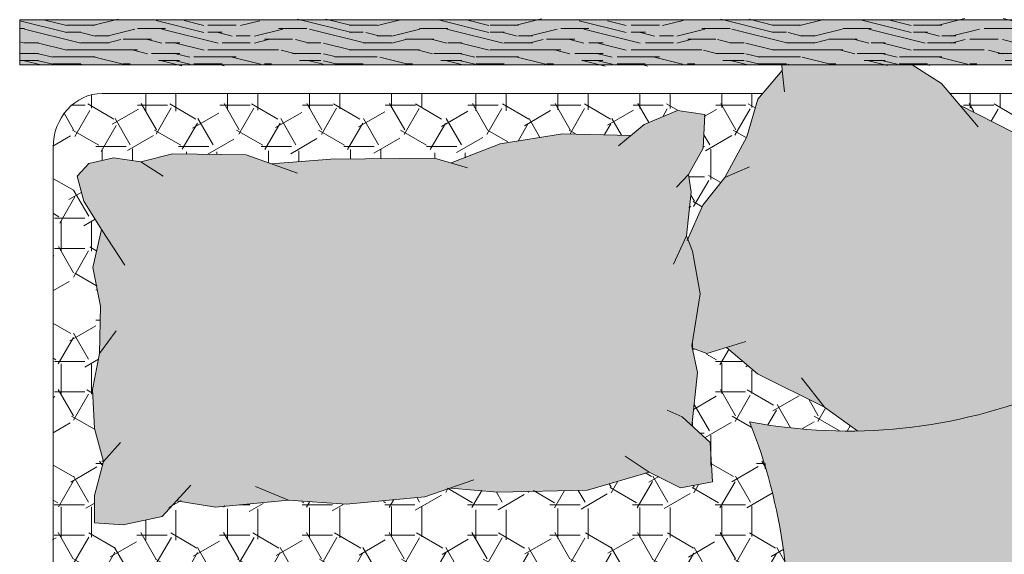
# Model space of a CAD drawing. Units: inches. Extents: x 1994 to 3075, y 3517 to 3950.
# Tile 44 of 58: x 1994.62902 to 1994.66748, y 3553.75542 to 3553.77632. Entities that reach past the tile are written whole.
import ezdxf

# ---------------------------------------------------------------- set-up
doc = ezdxf.new("R2010")
doc.units = ezdxf.units.IN
doc.layers.add('A-FURN-REFR', color=8, linetype='Continuous', lineweight=13)
doc.layers.add('A-FURN-REFR-PATT', color=8, linetype='Continuous', lineweight=13)

msp = doc.modelspace()

# ---------------------------------------------------------------- hatches: boundary and pattern name
at = {"layer": 'A-FURN-REFR-PATT'}
msp.add_hatch(color=256, dxfattribs=at).paths.add_polyline_path([(1994.683555, 3553.776316), (1994.629017, 3553.776316), (1994.629017, 3553.774549), (1994.683555, 3553.774549)])
h = msp.add_hatch(dxfattribs=at)
h.set_pattern_fill('LEGNO1', color=256, scale=0.005512, style=0, pattern_type=2)
h.set_pattern_definition([(0, (2000.7131367, 3549.9540566), (0, 0.005511811), [0.0011023622, -0.0016535433, 0.000551181, -0.0022047244]), (0, (2000.716995, 3549.9541944), (0, 0.005511811), [0.001102362, -0.004409449]), (0, (2000.716444, 3549.95447), (0, 0.005511811), [0.000551181, -0.00496063]), (0, (2000.713412, 3549.954608), (0, 0.005511811), [0.0002755906, -0.0038582677, 0.0002755906, -0.0011023622]), (0, (2000.7153414, 3549.9548834), (0, 0.005511811), [0.0011023622, -0.0016535433, 0.0002755906, -0.002480315]), (0, (2000.7139634, 3549.955021), (0, 0.005511811), [0.0008267717, -0.0046850394]), (0, (2000.7153414, 3549.955159), (0, 0.005511811), [0.0016535433, -0.0038582677]), (0, (2000.713688, 3549.955297), (0, 0.005511811), [0.001102362, -0.004409449]), (0, (2000.7158926, 3549.9554346), (0, 0.005511811), [0.0027559055, -0.0027559055]), (0, (2000.714239, 3549.95571), (0, 0.005511811), [0.000551181, -0.0016535433, 0.0011023622, -0.0022047244]), (0, (2000.7180973, 3549.955848), (0, 0.005511811), [0.001102362, -0.004409449]), (0, (2000.716995, 3549.955986), (0, 0.005511811), [0.000551181, -0.00496063]), (0, (2000.7158926, 3549.9561236), (0, 0.005511811), [0.000551181, -0.00496063]), (0, (2000.7131367, 3549.9562614), (0, 0.005511811), [0.001102362, -0.004409449]), (0, (2000.7158926, 3549.956399), (0, 0.005511811), [0.001102362, -0.004409449]), (0, (2000.7158926, 3549.956675), (0, 0.005511811), [0.0011023622, -0.0011023622, 0.0011023622, -0.0022047244]), (0, (2000.71479, 3549.9569503), (0, 0.005511811), [0.000551181, -0.0027559055, 0.0011023622, -0.0011023622]), (0, (2000.7158926, 3549.957088), (0, 0.005511811), [0.0016535433, -0.0038582677]), (0, (2000.7158926, 3549.957364), (0, 0.005511811), [0.001102362, -0.004409449]), (0, (2000.713688, 3549.9575015), (0, 0.005511811), [0.0016535433, -0.0022047244, 0.000551181, -0.0011023622]), (0, (2000.713688, 3549.957777), (0, 0.005511811), [0.0027559055, -0.0027559055]), (0, (2000.716995, 3549.957915), (0, 0.005511811), [0.000551181, -0.00496063]), (0, (2000.7153414, 3549.9580527), (0, 0.005511811), [0.001102362, -0.004409449]), (0, (2000.714239, 3549.9581905), (0, 0.005511811), [0.000551181, -0.0022047244, 0.000551181, -0.0022047244]), (0, (2000.713688, 3549.9583283), (0, 0.005511811), [0.000551181, -0.0016535433, 0.0011023622, -0.0022047244]), (0, (2000.71479, 3549.958466), (0, 0.005511811), [0.000551181, -0.0027559055, 0.000551181, -0.0016535433]), (0, (2000.7158926, 3549.958604), (0, 0.005511811), [0.0016535433, -0.0038582677]), (0, (2000.713688, 3549.9588795), (0, 0.005511811), [0.001102362, -0.004409449]), (0, (2000.716444, 3549.959017), (0, 0.005511811), [0.000551181, -0.00496063]), (0, (2000.717546, 3549.959155), (0, 0.005511811), [0.000551181, -0.00496063]), (14.036243, (2000.7169949, 3549.95447), (0.00551181102, -2e-13), [0.0005677165, -0.022158062]), (14.036243, (2000.7175461, 3549.9557102), (0.00551181102, -2e-13), [0.0005677165, -0.022158062]), (14.036243, (2000.7169949, 3549.9590173), (0.00551181102, -2e-13), [0.0005677165, -0.022158062]), (14.036243, (2000.7153414, 3549.9569503), (0.00551181102, -2e-13), [0.0005677165, -0.022158062]), (14.036243, (2000.7164437, 3549.9577771), (0.00551181102, -2e-13), [0.0005677165, -0.022158062]), (14.036243, (2000.7169949, 3549.9573637), (0.00551181102, -2e-13), [0.0005677165, -0.022158062]), (14.036243, (2000.714239, 3549.9583283), (0.00551181102, -2e-13), [0.0005677165, -0.022158062]), (14.036243, (2000.7164437, 3549.9580527), (0.00551181102, -2e-13), [0.0005677165, -0.022158062]), (14.036243, (2000.7175461, 3549.9559858), (0.00551181102, -2e-13), [0.001135433, -0.0215903454]), (14.036243, (2000.7169949, 3549.9563992), (0.00551181102, -2e-13), [0.001135433, -0.0215903454]), (14.036243, (2000.7169949, 3549.9566748), (0.00551181102, -2e-13), [0.001135433, -0.0215903454]), (165.963757, (2000.7153414, 3549.9548834), (-0.00551181102, -2e-13), [0.0005677165, -0.001135433, 0.0005677165, -0.0204549123]), (165.963757, (2000.714239, 3549.9557102), (-0.00551181102, -2e-13), [0.0005677165, -0.022158062]), (165.963757, (2000.714239, 3549.9581905), (-0.00551181102, -2e-13), [0.001135433, -0.0215903454]), (194.036243, (2000.7169949, 3549.9541944), (-0.00551181102, 2e-13), [0.0005677165, -0.022158062]), (345.963757, (2000.7180973, 3549.9541944), (0.00551181102, 2e-13), [0.0005677165, -0.022158062]), (345.963757, (2000.7164437, 3549.9561236), (0.00551181102, 2e-13), [0.0005677165, -0.022158062]), (345.963757, (2000.7175461, 3549.9570881), (0.00551181102, 2e-13), [0.0005677165, -0.022158062]), (345.963757, (2000.7153414, 3549.9575015), (0.00551181102, 2e-13), [0.0005677165, -0.022158062]), (345.963757, (2000.7147902, 3549.9581905), (0.00551181102, 2e-13), [0.0005677165, -0.022158062]), (345.963757, (2000.7153414, 3549.9584661), (0.00551181102, 2e-13), [0.0005677165, -0.022158062]), (345.963757, (2000.7153414, 3549.9575015), (0.00551181102, 2e-13), [0.0005677165, -0.022158062]), (345.963757, (2000.7169949, 3549.9583283), (0.00551181102, 2e-13), [0.002270866, -0.0204549123]), (345.963757, (2000.7136878, 3549.9546078), (0.00551181102, 2e-13), [0.002270866, -0.0204549123]), (345.963757, (2000.714239, 3549.9550212), (0.00551181102, 2e-13), [0.002270866, -0.0204549123]), (345.963757, (2000.7147902, 3549.9552968), (0.00551181102, 2e-13), [0.0005677165, -0.001135433, 0.001135433, -0.0198871958]), (345.963757, (2000.7147902, 3549.9557102), (0.00551181102, 2e-13), [0.001135433, -0.001135433, 0.001135433, -0.0193194793]), (345.963757, (2000.714239, 3549.9562614), (0.00551181102, 2e-13), [0.002270866, -0.0204549123]), (345.963757, (2000.7136878, 3549.9566748), (0.00551181102, 2e-13), [0.002270866, -0.0204549123]), (345.963757, (2000.7136878, 3549.9569503), (0.00551181102, 2e-13), [0.002270866, -0.0204549123]), (345.963757, (2000.7175461, 3549.9586039), (0.00551181102, 2e-13), [0.0005677165, -0.022158062]), (345.963768, (2000.7180973, 3549.959155), (0.00551181102, 1.06e-09), [0.001135433, -0.0215903454]), (345.963768, (2000.7147902, 3549.9588795), (0.00551181102, 1.06e-09), [0.001135433, -0.0215903454]), (345.963758, (2000.714239, 3549.9540566), (0.00551181102, 1e-10), [0.002270866, -0.0204549123]), (345.963758, (2000.7175461, 3549.9579149), (0.00551181102, 1e-10), [0.0017031496, -0.021022629]), (345.963758, (2000.7180973, 3549.9575015), (0.00551181102, 1e-10), [0.0034062992, -0.0193194793])])
h.paths.add_polyline_path([(1994.683555, 3553.776316), (1994.629017, 3553.776316), (1994.629017, 3553.774549), (1994.683555, 3553.774549)])
h = msp.add_hatch(color=256, dxfattribs=at)
h.set_gradient(color1=(238, 215, 180), color2=(243, 226, 201), one_color=1, tint=0.87)
edge = h.paths.add_edge_path()
edge.add_line((1994.676159, 3553.76789), (1994.673866, 3553.768856))
edge.add_line((1994.673866, 3553.768856), (1994.671861, 3553.769242))
edge.add_line((1994.671861, 3553.769242), (1994.671387, 3553.769751))
edge.add_line((1994.671387, 3553.769751), (1994.66783, 3553.771902))
edge.add_line((1994.66783, 3553.771902), (1994.665734, 3553.77298))
edge.add_line((1994.665734, 3553.77298), (1994.665027, 3553.773822))
edge.add_line((1994.665027, 3553.773822), (1994.663884, 3553.774549))
edge.add_line((1994.663884, 3553.774549), (1994.658782, 3553.774549))
edge.add_line((1994.658782, 3553.774549), (1994.6588, 3553.774326))
edge.add_line((1994.6588, 3553.774326), (1994.657844, 3553.773215))
edge.add_line((1994.657844, 3553.773215), (1994.657423, 3553.771734))
edge.add_line((1994.657423, 3553.771734), (1994.656565, 3553.770145))
edge.add_line((1994.656565, 3553.770145), (1994.655702, 3553.76907))
edge.add_line((1994.655702, 3553.76907), (1994.655113, 3553.767736))
edge.add_line((1994.655113, 3553.767736), (1994.6553, 3553.767274))
edge.add_line((1994.6553, 3553.767274), (1994.655602, 3553.765604))
edge.add_line((1994.655602, 3553.765604), (1994.655292, 3553.763679))
edge.add_line((1994.655292, 3553.763679), (1994.655292, 3553.76348))
edge.add_line((1994.655292, 3553.76348), (1994.655293, 3553.763476))
edge.add_line((1994.655293, 3553.763476), (1994.655861, 3553.763272))
edge.add_line((1994.655861, 3553.763272), (1994.656621, 3553.763504))
edge.add_line((1994.656621, 3553.763504), (1994.657839, 3553.762473))
edge.add_line((1994.657839, 3553.762473), (1994.660448, 3553.761168))
edge.add_line((1994.660448, 3553.761168), (1994.661753, 3553.760238))
edge.add_ellipse((1994.661382, 3553.784799), major_axis=(0, 0.024564), ratio=0.910403, start_angle=180.8636, end_angle=184.4499)
edge.add_ellipse((1994.661382, 3553.784799), major_axis=(0, 0.024564), ratio=0.910403, start_angle=184.4499, end_angle=194.365)
edge.add_ellipse((1994.661382, 3553.784799), major_axis=(0, 0.024564), ratio=0.910403, start_angle=194.365, end_angle=199.1151)
edge.add_ellipse((1994.691382, 3553.757287), major_axis=(0, 0.024638), ratio=0.910403, start_angle=78.3263, end_angle=85.2271)
edge.add_ellipse((1994.691382, 3553.757287), major_axis=(0, 0.024638), ratio=0.910403, start_angle=85.2271, end_angle=92.5166)
edge.add_line((1994.66897, 3553.756302), (1994.670799, 3553.755226))
edge.add_line((1994.670799, 3553.755226), (1994.673214, 3553.754537))
edge.add_line((1994.673214, 3553.754537), (1994.674009, 3553.753346))
edge.add_line((1994.674009, 3553.753346), (1994.675202, 3553.75288))
edge.add_line((1994.675202, 3553.75288), (1994.675812, 3553.754261))
edge.add_line((1994.675812, 3553.754261), (1994.675477, 3553.755213))
edge.add_line((1994.675477, 3553.755213), (1994.676595, 3553.756914))
edge.add_line((1994.676595, 3553.756914), (1994.67687, 3553.757942))
edge.add_line((1994.67687, 3553.757942), (1994.678066, 3553.759541))
edge.add_line((1994.678066, 3553.759541), (1994.678548, 3553.76116))
edge.add_line((1994.678548, 3553.76116), (1994.678603, 3553.761813))
edge.add_line((1994.678603, 3553.761813), (1994.679525, 3553.763197))
edge.add_line((1994.679525, 3553.763197), (1994.679737, 3553.763852))
edge.add_line((1994.679737, 3553.763852), (1994.680539, 3553.764349))
edge.add_line((1994.680539, 3553.764349), (1994.680823, 3553.764661))
edge.add_line((1994.680823, 3553.764661), (1994.681343, 3553.765554))
edge.add_line((1994.681343, 3553.765554), (1994.680491, 3553.766264))
edge.add_line((1994.680491, 3553.766264), (1994.679113, 3553.766487))
edge.add_line((1994.679113, 3553.766487), (1994.67846, 3553.766389))
edge.add_line((1994.67846, 3553.766389), (1994.676159, 3553.76789))
h = msp.add_hatch(dxfattribs=at)
h.set_pattern_fill('ESA_QT1', color=256, scale=0.001181, style=0, pattern_type=2)
h.set_pattern_definition([(0, (2000.7131367, 3549.95567), (0.0016133858, 0.0027944882), [0.0011811024, -0.0020457874]), (0, (2000.7131367, 3549.956851), (0.0016133858, 0.0027944882), [0.0011811024, -0.0020457874]), (60, (2000.7147507, 3549.9540566), (-0.0016134048, 0.0027944772), [0.0011811024, -0.0020457874]), (60, (2000.7137272, 3549.9546472), (-0.0016134048, 0.0027944772), [0.0011811024, -0.0020457874]), (120, (2000.7159311, 3549.9540566), (-0.0032267907, -1.1e-08), [0.0011811024, -0.0020457874]), (120, (2000.716954, 3549.9546472), (-0.0032267907, -1.1e-08), [0.0011811024, -0.0020457874]), (90, (2000.7131367, 3549.95567), (-0.00161338583, 0.0027944882), [0.0011811024, -0.0044079921]), (90, (2000.7143178, 3549.95567), (-0.00161338583, 0.0027944882), [0.0011811024, -0.0044079921]), (30, (2000.7159311, 3549.9540566), (0.00161340485, 0.0027944772), [0.0011811024, -0.0044079921]), (150, (2000.71475, 3549.9540566), (-0.00322679068, 1.1e-08), [0.0011811024, -0.0044079921]), (30, (2000.7153406, 3549.9550795), (0.00161340485, 0.0027944772), [0.0011811024, -0.0044079921]), (150, (2000.7153406, 3549.9550795), (-0.00322679068, 1.1e-08), [0.0011811024, -0.0044079921])])
edge = h.paths.add_edge_path()
edge.add_ellipse((1994.640876, 3553.752584), major_axis=(0, 0.019971), ratio=0.910403, start_angle=279.2385, end_angle=295.7126)
edge.add_ellipse((1994.661382, 3553.784799), major_axis=(0, 0.024564), ratio=0.910403, start_angle=170.9484, end_angle=180.8636)
edge.add_line((1994.661753, 3553.760238), (1994.660448, 3553.761168))
edge.add_line((1994.660448, 3553.761168), (1994.657839, 3553.762473))
edge.add_line((1994.657839, 3553.762473), (1994.656621, 3553.763504))
edge.add_line((1994.656621, 3553.763504), (1994.655861, 3553.763272))
edge.add_line((1994.655861, 3553.763272), (1994.655293, 3553.763476))
edge.add_line((1994.655293, 3553.763476), (1994.655493, 3553.762522))
edge.add_line((1994.655493, 3553.762522), (1994.655292, 3553.760584))
edge.add_line((1994.655292, 3553.760584), (1994.655292, 3553.760424))
edge.add_line((1994.655292, 3553.760424), (1994.655994, 3553.759788))
edge.add_line((1994.655994, 3553.759788), (1994.656079, 3553.758256))
edge.add_line((1994.656079, 3553.758256), (1994.654831, 3553.75802))
edge.add_line((1994.654831, 3553.75802), (1994.653607, 3553.75863))
edge.add_line((1994.653607, 3553.75863), (1994.651194, 3553.757931))
edge.add_line((1994.651194, 3553.757931), (1994.647697, 3553.757851))
edge.add_line((1994.647697, 3553.757851), (1994.645839, 3553.758008))
edge.add_line((1994.645839, 3553.758008), (1994.644836, 3553.757661))
edge.add_line((1994.644836, 3553.757661), (1994.64177, 3553.757379))
edge.add_line((1994.64177, 3553.757379), (1994.63952, 3553.757537))
edge.add_line((1994.63952, 3553.757537), (1994.636664, 3553.757269))
edge.add_line((1994.636664, 3553.757269), (1994.635142, 3553.757511))
edge.add_line((1994.635142, 3553.757511), (1994.634583, 3553.7569))
edge.add_line((1994.634583, 3553.7569), (1994.633061, 3553.756568))
edge.add_line((1994.633061, 3553.756568), (1994.631936, 3553.756647))
edge.add_line((1994.631936, 3553.756647), (1994.631946, 3553.757723))
edge.add_line((1994.631946, 3553.757723), (1994.632293, 3553.759053))
edge.add_line((1994.632293, 3553.759053), (1994.631942, 3553.760336))
edge.add_line((1994.631942, 3553.760336), (1994.631857, 3553.761868))
edge.add_line((1994.631857, 3553.761868), (1994.63213, 3553.76327))
edge.add_line((1994.63213, 3553.76327), (1994.632168, 3553.765117))
edge.add_line((1994.632168, 3553.765117), (1994.631874, 3553.766635))
edge.add_line((1994.631874, 3553.766635), (1994.632212, 3553.768118))
edge.add_line((1994.632212, 3553.768118), (1994.631521, 3553.769225))
edge.add_line((1994.631521, 3553.769225), (1994.631256, 3553.770206))
edge.add_line((1994.631256, 3553.770206), (1994.631719, 3553.770698))
edge.add_line((1994.631719, 3553.770698), (1994.632688, 3553.770917))
edge.add_line((1994.632688, 3553.770917), (1994.633747, 3553.770757))
edge.add_line((1994.633747, 3553.770757), (1994.63499, 3553.77107))
edge.add_line((1994.63499, 3553.77107), (1994.637864, 3553.771031))
edge.add_line((1994.637864, 3553.771031), (1994.638857, 3553.770678))
edge.add_line((1994.638857, 3553.770678), (1994.641165, 3553.770867))
edge.add_line((1994.641165, 3553.770867), (1994.645224, 3553.770907))
edge.add_line((1994.645224, 3553.770907), (1994.645865, 3553.770719))
edge.add_line((1994.645865, 3553.770719), (1994.647785, 3553.771462))
edge.add_line((1994.647785, 3553.771462), (1994.650215, 3553.771855))
edge.add_line((1994.650215, 3553.771855), (1994.65289, 3553.771785))
edge.add_line((1994.65289, 3553.771785), (1994.653416, 3553.772222))
edge.add_line((1994.653416, 3553.772222), (1994.654716, 3553.77277))
edge.add_line((1994.654716, 3553.77277), (1994.655776, 3553.77261))
edge.add_line((1994.655776, 3553.77261), (1994.655708, 3553.771299))
edge.add_line((1994.655708, 3553.771299), (1994.655135, 3553.770261))
edge.add_line((1994.655135, 3553.770261), (1994.655243, 3553.769577))
edge.add_line((1994.655243, 3553.769577), (1994.655057, 3553.767873))
edge.add_line((1994.655057, 3553.767873), (1994.655113, 3553.767736))
edge.add_line((1994.655113, 3553.767736), (1994.655702, 3553.76907))
edge.add_line((1994.655702, 3553.76907), (1994.656565, 3553.770145))
edge.add_line((1994.656565, 3553.770145), (1994.657423, 3553.771734))
edge.add_line((1994.657423, 3553.771734), (1994.657844, 3553.773215))
edge.add_line((1994.657844, 3553.773215), (1994.658028, 3553.77343))
edge.add_line((1994.658028, 3553.77343), (1994.632244, 3553.77343))
edge.add_ellipse((1994.632244, 3553.771319), major_axis=(0, 0.002111), ratio=0.910403, start_angle=0, end_angle=90)
edge.add_line((1994.630322, 3553.771319), (1994.630322, 3553.749441))
edge.add_line((1994.630322, 3553.749441), (1994.637709, 3553.750433))
edge.add_line((1994.637709, 3553.750433), (1994.645849, 3553.752088))
edge.add_line((1994.645849, 3553.752088), (1994.649254, 3553.75227))
edge.add_line((1994.649254, 3553.75227), (1994.654398, 3553.752423))
edge.add_line((1994.654398, 3553.752423), (1994.656593, 3553.752621))
edge.add_ellipse((1994.639937, 3553.760628), major_axis=(0, 0.019971), ratio=0.910403, start_angle=244.323, end_angle=253.1594)
edge.add_ellipse((1994.674344, 3553.771437), major_axis=(0, 0.024564), ratio=0.910403, start_angle=133.6721, end_angle=139.6806)
edge.add_line((1994.659095, 3553.753469), (1994.658861, 3553.755509))
edge = h.paths.add_edge_path()
edge.add_ellipse((1994.680284, 3553.771319), major_axis=(0, 0.002111), ratio=0.910403, start_angle=270, end_angle=360)
edge.add_line((1994.680284, 3553.77343), (1994.665356, 3553.77343))
edge.add_line((1994.665356, 3553.77343), (1994.665734, 3553.77298))
edge.add_line((1994.665734, 3553.77298), (1994.66783, 3553.771902))
edge.add_line((1994.66783, 3553.771902), (1994.671387, 3553.769751))
edge.add_line((1994.671387, 3553.769751), (1994.671861, 3553.769242))
edge.add_line((1994.671861, 3553.769242), (1994.673866, 3553.768856))
edge.add_line((1994.673866, 3553.768856), (1994.676159, 3553.76789))
edge.add_line((1994.676159, 3553.76789), (1994.67846, 3553.766389))
edge.add_line((1994.67846, 3553.766389), (1994.679113, 3553.766487))
edge.add_line((1994.679113, 3553.766487), (1994.680491, 3553.766264))
edge.add_line((1994.680491, 3553.766264), (1994.681343, 3553.765554))
edge.add_line((1994.681343, 3553.765554), (1994.680699, 3553.764448))
edge.add_line((1994.680699, 3553.764448), (1994.679737, 3553.763852))
edge.add_line((1994.679737, 3553.763852), (1994.679525, 3553.763197))
edge.add_line((1994.679525, 3553.763197), (1994.678603, 3553.761813))
edge.add_line((1994.678603, 3553.761813), (1994.678548, 3553.76116))
edge.add_line((1994.678548, 3553.76116), (1994.678066, 3553.759541))
edge.add_line((1994.678066, 3553.759541), (1994.676936, 3553.75803))
edge.add_line((1994.676936, 3553.75803), (1994.676848, 3553.757857))
edge.add_line((1994.676848, 3553.757857), (1994.676595, 3553.756914))
edge.add_line((1994.676595, 3553.756914), (1994.675477, 3553.755213))
edge.add_line((1994.675477, 3553.755213), (1994.675812, 3553.754261))
edge.add_line((1994.675812, 3553.754261), (1994.675202, 3553.75288))
edge.add_line((1994.675202, 3553.75288), (1994.674009, 3553.753346))
edge.add_line((1994.674009, 3553.753346), (1994.673214, 3553.754537))
edge.add_line((1994.673214, 3553.754537), (1994.670799, 3553.755226))
edge.add_line((1994.670799, 3553.755226), (1994.66897, 3553.756302))
edge.add_ellipse((1994.691382, 3553.757287), major_axis=(0, 0.024638), ratio=0.910403, start_angle=92.5166, end_angle=102.9728)
edge.add_line((1994.66943, 3553.75223), (1994.673814, 3553.75171))
edge.add_line((1994.673814, 3553.75171), (1994.677653, 3553.751587))
edge.add_line((1994.677653, 3553.751587), (1994.682205, 3553.751587))
edge.add_line((1994.682205, 3553.751587), (1994.682205, 3553.755102))
edge.add_line((1994.682205, 3553.755102), (1994.682205, 3553.771319))
h = msp.add_hatch(color=256, dxfattribs=at)
h.set_gradient(color1=(238, 215, 180), color2=(243, 226, 201), one_color=1, tint=0.87)
h.paths.add_polyline_path([(1994.631936, 3553.756647), (1994.631946, 3553.757723), (1994.632293, 3553.759053), (1994.631942, 3553.760336), (1994.631857, 3553.761868), (1994.63213, 3553.76327), (1994.632168, 3553.765117), (1994.631874, 3553.766635), (1994.632212, 3553.768118), (1994.631521, 3553.769225), (1994.631256, 3553.770206), (1994.631719, 3553.770698), (1994.632688, 3553.770917), (1994.633747, 3553.770757), (1994.63499, 3553.77107), (1994.637864, 3553.771031), (1994.638857, 3553.770678), (1994.641165, 3553.770867), (1994.645224, 3553.770907), (1994.645865, 3553.770719), (1994.647785, 3553.771462), (1994.650215, 3553.771855), (1994.65289, 3553.771785), (1994.653416, 3553.772222), (1994.654716, 3553.77277), (1994.655776, 3553.77261), (1994.655708, 3553.771299), (1994.655135, 3553.770261), (1994.655243, 3553.769577), (1994.655057, 3553.767873), (1994.6553, 3553.767274), (1994.655602, 3553.765604), (1994.655261, 3553.763487), (1994.655293, 3553.763476), (1994.655493, 3553.762522), (1994.655277, 3553.760438), (1994.655994, 3553.759788), (1994.656079, 3553.758256), (1994.654831, 3553.75802), (1994.653607, 3553.75863), (1994.651194, 3553.757931), (1994.647697, 3553.757851), (1994.645839, 3553.758008), (1994.644836, 3553.757661), (1994.64177, 3553.757379), (1994.63952, 3553.757537), (1994.636664, 3553.757269), (1994.635142, 3553.757511), (1994.634583, 3553.7569), (1994.633061, 3553.756568)])
h = msp.add_hatch(color=256, dxfattribs=at)
h.set_gradient(color1=(223, 184, 155), color2=(248, 239, 232), one_color=1, tint=0.94, name='SPHERICAL')
edge = h.paths.add_edge_path()
edge.add_ellipse((1994.691382, 3553.757287), major_axis=(0, 0.024638), ratio=0.910403, start_angle=92.5166, end_angle=102.9728, ccw=False)
edge.add_ellipse((1994.691382, 3553.757287), major_axis=(0, 0.024638), ratio=0.910403, start_angle=78.3263, end_angle=92.5166, ccw=False)
edge.add_ellipse((1994.661382, 3553.784799), major_axis=(0, 0.024564), ratio=0.910403, start_angle=180.8636, end_angle=199.1151, ccw=False)
edge.add_ellipse((1994.661382, 3553.784799), major_axis=(0, 0.024564), ratio=0.910403, start_angle=170.9484, end_angle=180.8636, ccw=False)
edge.add_ellipse((1994.640876, 3553.752584), major_axis=(0, 0.019971), ratio=0.910403, start_angle=279.2385, end_angle=295.7126, ccw=False)
edge.add_line((1994.658861, 3553.755509), (1994.659095, 3553.753469))
edge.add_ellipse((1994.674344, 3553.771437), major_axis=(0, 0.024564), ratio=0.910403, start_angle=139.6806, end_angle=157.0382)
edge.add_ellipse((1994.66794, 3553.708563), major_axis=(0, 0.04074), ratio=0.910403, start_angle=356.8603, end_angle=364.2706, ccw=False)
edge.add_line((1994.670171, 3553.749229), (1994.670182, 3553.749241))
edge.add_ellipse((1994.691382, 3553.757287), major_axis=(0, 0.024638), ratio=0.910403, start_angle=102.9728, end_angle=110.7835, ccw=False)

# ---------------------------------------------------------------- linework, layer by layer
at = {"layer": 'A-FURN-REFR'}
for p, q in [((1994.629017, 3553.776316), (1994.629017, 3553.774549)), ((1994.683555, 3553.776316), (1994.629017, 3553.776316)), ((1994.629017, 3553.774549), (1994.683555, 3553.774549)), ((1994.658782, 3553.774549), (1994.6588, 3553.774326)), ((1994.663884, 3553.774549), (1994.665027, 3553.773822)), ((1994.6588, 3553.774326), (1994.657844, 3553.773215)), ((1994.6588, 3553.774326), (1994.658885, 3553.773497)), ((1994.665027, 3553.773822), (1994.666452, 3553.772125)), ((1994.632244, 3553.77343), (1994.658028, 3553.77343)), ((1994.665356, 3553.77343), (1994.680284, 3553.77343)), ((1994.657844, 3553.773215), (1994.657423, 3553.771734)), ((1994.665734, 3553.77298), (1994.66783, 3553.771902)), ((1994.654716, 3553.77277), (1994.653416, 3553.772222)), ((1994.655776, 3553.77261), (1994.654716, 3553.77277)), ((1994.655708, 3553.771299), (1994.655776, 3553.77261)), ((1994.653416, 3553.772222), (1994.652411, 3553.771386)), ((1994.647785, 3553.771462), (1994.650215, 3553.771855)), ((1994.650215, 3553.771855), (1994.65289, 3553.771785)), ((1994.657423, 3553.771734), (1994.656565, 3553.770145)), ((1994.645865, 3553.770719), (1994.647785, 3553.771462)), ((1994.630322, 3553.749441), (1994.630322, 3553.771319)), ((1994.633747, 3553.770757), (1994.63499, 3553.77107)), ((1994.63499, 3553.77107), (1994.637864, 3553.771031)), ((1994.637864, 3553.771031), (1994.639864, 3553.770319)), ((1994.655135, 3553.770261), (1994.655708, 3553.771299)), ((1994.631719, 3553.770698), (1994.631256, 3553.770206)), ((1994.632688, 3553.770917), (1994.631719, 3553.770698)), ((1994.633747, 3553.770757), (1994.632688, 3553.770917)), ((1994.633747, 3553.770757), (1994.634618, 3553.7702)), ((1994.638857, 3553.770678), (1994.641165, 3553.770867)), ((1994.641165, 3553.770867), (1994.645224, 3553.770907)), ((1994.645224, 3553.770907), (1994.646506, 3553.770531)), ((1994.631256, 3553.770206), (1994.631521, 3553.769225)), ((1994.654672, 3553.769769), (1994.655135, 3553.770261)), ((1994.655243, 3553.769577), (1994.655135, 3553.770261)), ((1994.657529, 3553.770569), (1994.656565, 3553.770145)), ((1994.656565, 3553.770145), (1994.655702, 3553.76907)), ((1994.655057, 3553.767873), (1994.655243, 3553.769577)), ((1994.631521, 3553.769225), (1994.632212, 3553.768118)), ((1994.655702, 3553.76907), (1994.655092, 3553.767689)), ((1994.632212, 3553.768118), (1994.631874, 3553.766635)), ((1994.632212, 3553.768118), (1994.63313, 3553.766719)), ((1994.654558, 3553.766764), (1994.655057, 3553.767873)), ((1994.6553, 3553.767274), (1994.655057, 3553.767873)), ((1994.655602, 3553.765604), (1994.6553, 3553.767274)), ((1994.631874, 3553.766635), (1994.632168, 3553.765117)), ((1994.655274, 3553.763567), (1994.655602, 3553.765604)), ((1994.632168, 3553.765117), (1994.63213, 3553.76327)), ((1994.632781, 3553.764159), (1994.63213, 3553.76327)), ((1994.655292, 3553.76348), (1994.655292, 3553.763679)), ((1994.655861, 3553.763272), (1994.657387, 3553.763737)), ((1994.63213, 3553.76327), (1994.631857, 3553.761868)), ((1994.655493, 3553.762522), (1994.655274, 3553.763567)), ((1994.655293, 3553.763476), (1994.655861, 3553.763272)), ((1994.656621, 3553.763504), (1994.657839, 3553.762473)), ((1994.655277, 3553.760438), (1994.655493, 3553.762522)), ((1994.657839, 3553.762473), (1994.660448, 3553.761168)), ((1994.65956, 3553.762324), (1994.660448, 3553.761168)), ((1994.631857, 3553.761868), (1994.631942, 3553.760336)), ((1994.654888, 3553.76079), (1994.654313, 3553.76106)), ((1994.660448, 3553.761168), (1994.661753, 3553.760238)), ((1994.655994, 3553.759788), (1994.654888, 3553.76079)), ((1994.655292, 3553.760424), (1994.655292, 3553.760584)), ((1994.631942, 3553.760336), (1994.632293, 3553.759053)), ((1994.632953, 3553.759789), (1994.632293, 3553.759053)), ((1994.656079, 3553.758256), (1994.655994, 3553.759788)), ((1994.632293, 3553.759053), (1994.631946, 3553.757723)), ((1994.652662, 3553.759258), (1994.653607, 3553.75863)), ((1994.644836, 3553.757661), (1994.64676, 3553.758327)), ((1994.651194, 3553.757931), (1994.653607, 3553.75863)), ((1994.653607, 3553.75863), (1994.654831, 3553.75802)), ((1994.634583, 3553.7569), (1994.635706, 3553.758128)), ((1994.63823, 3553.758066), (1994.63952, 3553.757537)), ((1994.645839, 3553.758008), (1994.647697, 3553.757851)), ((1994.647697, 3553.757851), (1994.651194, 3553.757931)), ((1994.654831, 3553.75802), (1994.656079, 3553.758256)), ((1994.631946, 3553.757723), (1994.631936, 3553.756647)), ((1994.635142, 3553.757511), (1994.636664, 3553.757269)), ((1994.636664, 3553.757269), (1994.63952, 3553.757537)), ((1994.63952, 3553.757537), (1994.64177, 3553.757379)), ((1994.64177, 3553.757379), (1994.644836, 3553.757661)), ((1994.633061, 3553.756568), (1994.634583, 3553.7569)), ((1994.631936, 3553.756647), (1994.633061, 3553.756568)), ((1994.658861, 3553.755509), (1994.659095, 3553.753469))]:
    msp.add_line(p, q, dxfattribs=at)
at = {"layer": 'A-FURN-REFR', "extrusion": (0, 0, -1)}
for centre, major_axis, start_param, end_param in [((1994.632244, 3553.771319), (0, 0.002111), 4.712389, 6.283185), ((1994.661382, 3553.784799), (0, 0.024564), 2.777849, 3.314824), ((1994.640876, 3553.752584), (0, 0.019971), 1.157636, 1.423784)]:
    msp.add_ellipse(centre, major_axis=major_axis, ratio=0.910403, start_param=start_param, end_param=end_param, dxfattribs=at)

doc.saveas('drawing.dxf')
